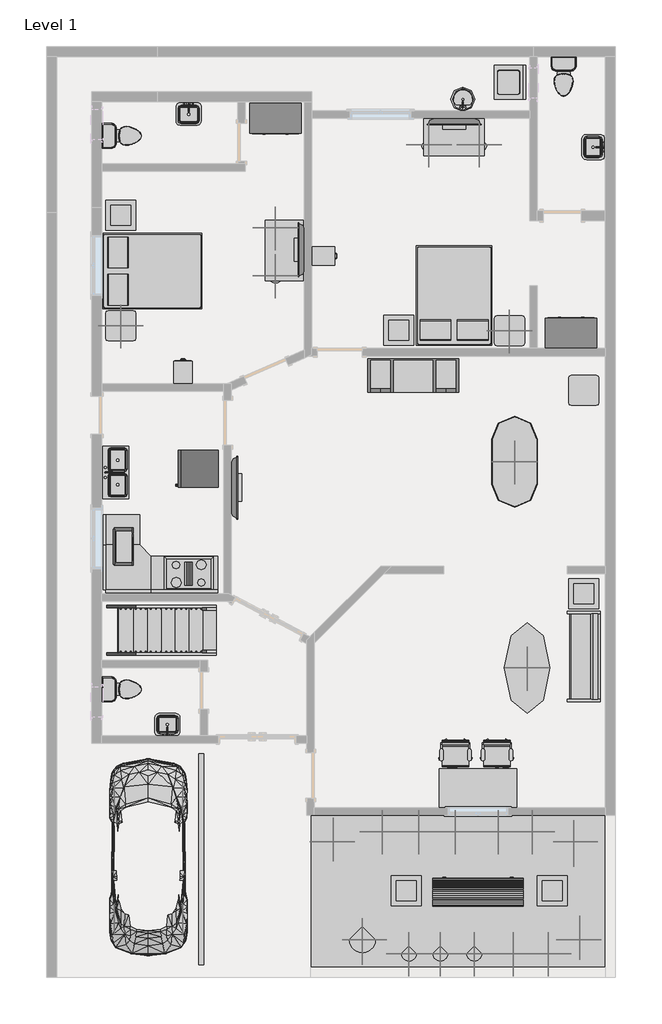
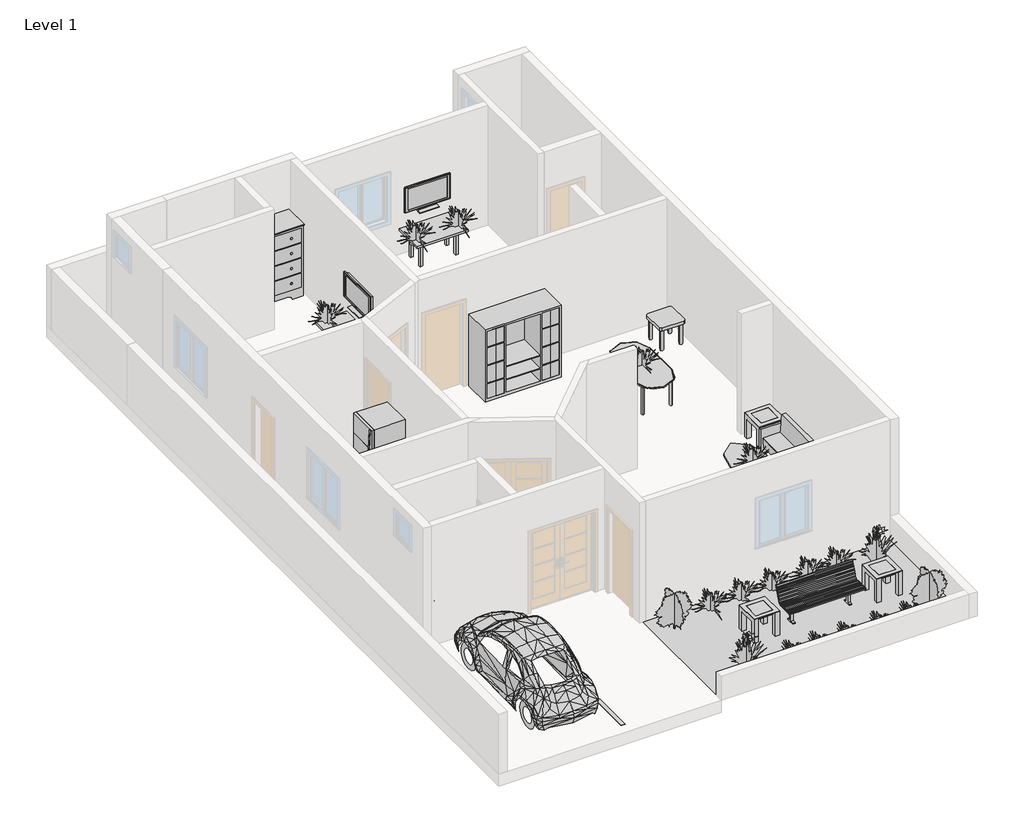
# One storey, part 2 of 2: 27 furniture elements, 23 geographic elements, 12 flow terminals, 7 proxies, 2 members, 2 railings, 1 stair flight.
"""IFC4 building model written with IfcOpenShell, lengths in millimetres."""

from ifc_helpers import new_model, si_unit, frame, origin, place, context, project, spatial, polyline, outline, extrude, triangles, transform, mapped, element, save
from components import proxy_bb1e6e30, proxy_8a8d5ab2, parking_space_9_x_18_90_deg_fdd9e8f5, rpc_beetle_rpc_beetle_3ce7ba48, proxy_a13a33b2, proxy_718fa39f, flow_terminal_accce45a, flow_terminal_a53be723, flow_terminal_d49f872f, flow_terminal_62a433f7, toilet_domestic_3d_toilet_domestic_3d_f7549cf7, toilet_domestic_3d_toilet_domestic_3d_183bbd19, furniture_1d2926bd, furniture_bb55ed6b, chair_task_arms_chair_task_arms_fa5a08ef, furniture_072f6425, furniture_f72bdee3, furniture_cf0b6580, furniture_a4ffab56, furniture_7a3aaa4f, furniture_fdf74506, furniture_b5c51a22, furniture_2c34a4f9, furniture_962d0db1, furniture_31d08a24, furniture_3f969c1c, furniture_b52c1e80, geographic_element_235d1464, rpc_plant_tropical_55f6ff97, rpc_plant_tropical_agave_1_5_93a2a214, rpc_plant_tropical_jungle_flame_3_9c4808c2, stair_flight_e425de01

model = new_model("IFC4")

# Units and contexts
model_context = context("Model", 3, world=origin())
ifc_project = project(units=[si_unit("LENGTHUNIT", "METRE", prefix="MILLI")], contexts=[model_context])

# Site, building, storey
site = spatial("IfcSite", under=ifc_project)
building = spatial("IfcBuilding", under=site)
storey = spatial("IfcBuildingStorey", under=building, Name="Level 1", Elevation=0.0)

# Proxies
placement = place(None, origin())
element("IfcBuildingElementProxy", 1, Name="Building Element Proxy", at=placement, inside=storey, context=model_context, shape_type="Tessellation", body=[
    triangles([(-7577.7508347, -2699.6256248, 0.0), (-7501.5508347, -5773.025528, 0.0), (-1557.950544, -5773.025528, 0.0), (-1557.950544, -2699.6256248, 0.0)], [[1, 2, 4], [3, 4, 2]], closed=False),
])
proxy_shape = proxy_bb1e6e30(model_context)
element("IfcBuildingElementProxy", 2, Name="Cook Top-4 Unit : 36\" x 20\"", ObjectType="Cook Top-4 Unit : 36\" x 20\"", at=placement, inside=storey, context=model_context, shape_type="MappedRepresentation", body=[
    mapped(proxy_shape, transform((-9965.3505662, 2175.4598603, 0.0), x_axis=(1.0, 0.0, 0.0), y_axis=(0.0, 1.0, 0.0), z_axis=(0.0, 0.0, 1.0))),
])
proxy_2_shape = proxy_8a8d5ab2(model_context)
element("IfcBuildingElementProxy", 3, Name="Microwave : 30\" x 16\" x 18\"", ObjectType="Microwave : 30\" x 16\" x 18\"", at=placement, inside=storey, context=model_context, shape_type="MappedRepresentation", body=[
    mapped(proxy_2_shape, transform((-11639.231072, 2222.1807348, 0.0), x_axis=(0.0, 1.0000000000000004, 0.0), y_axis=(-1.0000000000000004, 0.0, 0.0), z_axis=(0.0, 0.0, 1.0))),
])
parking_space_9_x_18_90_deg_shape = parking_space_9_x_18_90_deg_fdd9e8f5(model_context)
element("IfcBuildingElementProxy", 4, Name="Parking Space : 9' x 18' - 90 deg", ObjectType="Parking Space : 9' x 18' - 90 deg", at=placement, inside=storey, context=model_context, shape_type="MappedRepresentation", body=[
    mapped(parking_space_9_x_18_90_deg_shape, transform((-9711.3505662, -5722.2257293, 0.0), x_axis=(-1.0, 0.0, 0.0), y_axis=(0.0, -1.0, 0.0), z_axis=(0.0, 0.0, 1.0))),
])
rpc_beetle_rpc_beetle_shape = rpc_beetle_rpc_beetle_3ce7ba48(model_context)
element("IfcBuildingElementProxy", 5, Name="RPC Beetle : RPC Beetle", ObjectType="RPC Beetle : RPC Beetle", at=placement, inside=storey, context=model_context, shape_type="MappedRepresentation", body=[
    mapped(rpc_beetle_rpc_beetle_shape, transform((-10778.1505662, -4782.4257293, 0.0), x_axis=(1.0, 0.0, 0.0), y_axis=(0.0, 1.0, 0.0), z_axis=(0.0, 0.0, 1.0))),
])
proxy_3_shape = proxy_a13a33b2(model_context)
element("IfcBuildingElementProxy", 6, Name="Refrigerator : 30\" x 32\" RH", ObjectType="Refrigerator : 30\" x 32\" RH", at=placement, inside=storey, context=model_context, shape_type="MappedRepresentation", body=[
    mapped(proxy_3_shape, transform((-9754.2130662, 4296.8752993, 0.0), x_axis=(0.0, -1.0000000000000007, 0.0), y_axis=(1.0000000000000007, 0.0, 0.0), z_axis=(0.0, 0.0, 1.0))),
])
proxy_4_shape = proxy_718fa39f(model_context)
element("IfcBuildingElementProxy", 7, Name="Washer : 27\" x 25\" x 35\"", ObjectType="Washer : 27\" x 25\" x 35\"", at=placement, inside=storey, context=model_context, shape_type="MappedRepresentation", body=[
    mapped(proxy_4_shape, transform((-3754.800131, 12516.2917392, 0.0), x_axis=(0.0, -1.0000000000000004, 0.0), y_axis=(1.0000000000000004, 0.0, 0.0), z_axis=(0.0, 0.0, 1.0))),
])

# Flow terminals
flow_terminal_shape = flow_terminal_accce45a(model_context)
element("IfcFlowTerminal", 8, ObjectType="Floor Drain - Round : 5\" Strainer - 2\" Drain", at=placement, inside=storey, context=model_context, shape_type="MappedRepresentation", body=[
    mapped(flow_terminal_shape, transform((-10955.9505662, 11498.9742707, 0.0), x_axis=(1.0, 0.0, 0.0), y_axis=(0.0, 1.0, 0.0), z_axis=(0.0, 0.0, 1.0))),
])
element("IfcFlowTerminal", 9, ObjectType="Floor Drain - Round : 5\" Strainer - 2\" Drain", at=placement, inside=storey, context=model_context, shape_type="MappedRepresentation", body=[
    mapped(flow_terminal_shape, transform((-1938.9505662, 11727.5742707, 0.0), x_axis=(1.0, 0.0, 0.0), y_axis=(0.0, 1.0, 0.0), z_axis=(0.0, 0.0, 1.0))),
])
element("IfcFlowTerminal", 10, ObjectType="Floor Drain - Round : 5\" Strainer - 2\" Drain", at=placement, inside=storey, context=model_context, shape_type="MappedRepresentation", body=[
    mapped(flow_terminal_shape, transform((-11438.5505662, -743.8257293, 0.0), x_axis=(1.0, 0.0, 0.0), y_axis=(0.0, 1.0, 0.0), z_axis=(0.0, 0.0, 1.0))),
])
element("IfcFlowTerminal", 11, ObjectType="Floor Drain - Round : 5\" Strainer - 2\" Drain", at=placement, inside=storey, context=model_context, shape_type="MappedRepresentation", body=[
    mapped(flow_terminal_shape, transform((-4072.5505662, 12413.3742707, 0.0), x_axis=(1.0, 0.0, 0.0), y_axis=(0.0, 1.0, 0.0), z_axis=(0.0, 0.0, 1.0))),
])
flow_terminal_2_shape = flow_terminal_a53be723(model_context)
element("IfcFlowTerminal", 12, ObjectType="Sink Kitchen-Double : 42\" x 21\"", at=placement, inside=storey, context=model_context, shape_type="MappedRepresentation", body=[
    mapped(flow_terminal_2_shape, transform((-11436.2051651, 4204.4706197, 0.0), x_axis=(0.0, 1.0000000000000002, 0.0), y_axis=(-1.0000000000000002, 0.0, 0.0), z_axis=(0.0, 0.0, 1.0))),
])
flow_terminal_3_shape = flow_terminal_d49f872f(model_context)
element("IfcFlowTerminal", 13, ObjectType="Sink Vanity-Round : 19\" x 19\"", at=placement, inside=storey, context=model_context, shape_type="MappedRepresentation", body=[
    mapped(flow_terminal_3_shape, transform((-4331.4988256, 11839.263255, 0.0), x_axis=(-1.0000000000000004, 0.0, 0.0), y_axis=(0.0, -1.0000000000000004, 0.0), z_axis=(0.0, 0.0, 1.0))),
])
flow_terminal_4_shape = flow_terminal_62a433f7(model_context)
element("IfcFlowTerminal", 14, ObjectType="Sink Vanity-Square : 20\" x 18\"", at=placement, inside=storey, context=model_context, shape_type="MappedRepresentation", body=[
    mapped(flow_terminal_4_shape, transform((-9981.0398067, 11502.9788696, 0.0), x_axis=(1.0, 0.0, 0.0), y_axis=(0.0, 1.0, 0.0), z_axis=(0.0, 0.0, 1.0))),
])
element("IfcFlowTerminal", 15, ObjectType="Sink Vanity-Square : 20\" x 18\"", at=placement, inside=storey, context=model_context, shape_type="MappedRepresentation", body=[
    mapped(flow_terminal_4_shape, transform((-1750.7959673, 10803.4635113, 0.0), x_axis=(0.0, -1.0000000000000002, 0.0), y_axis=(1.0000000000000002, 0.0, 0.0), z_axis=(0.0, 0.0, 1.0))),
])
element("IfcFlowTerminal", 16, ObjectType="Sink Vanity-Square : 20\" x 18\"", at=placement, inside=storey, context=model_context, shape_type="MappedRepresentation", body=[
    mapped(flow_terminal_4_shape, transform((-10381.4613256, -919.2803281, 0.0), x_axis=(-1.0, 0.0, 0.0), y_axis=(0.0, -1.0, 0.0), z_axis=(0.0, 0.0, 1.0))),
])
toilet_domestic_3d_toilet_domestic_3d_shape = toilet_domestic_3d_toilet_domestic_3d_f7549cf7(model_context)
toilet_domestic_3d_toilet_domestic_3d_2_shape = toilet_domestic_3d_toilet_domestic_3d_183bbd19(model_context)
element("IfcFlowTerminal", 17, ObjectType="Toilet-Domestic-3D : Toilet-Domestic-3D", at=placement, inside=storey, context=model_context, shape_type="MappedRepresentation", body=[
    mapped(toilet_domestic_3d_toilet_domestic_3d_shape, transform((-11223.2545388, 11016.3742707, 0.0), x_axis=(0.0, 1.0, 0.0), y_axis=(-1.0, 0.0, 0.0), z_axis=(0.0, 0.0, 1.0))),
    mapped(toilet_domestic_3d_toilet_domestic_3d_2_shape, transform((-11223.2545388, 11016.3742707, 0.0), x_axis=(0.0, 1.0, 0.0), y_axis=(-1.0, 0.0, 0.0), z_axis=(0.0, 0.0, 1.0))),
])
element("IfcFlowTerminal", 18, ObjectType="Toilet-Domestic-3D : Toilet-Domestic-3D", at=placement, inside=storey, context=model_context, shape_type="MappedRepresentation", body=[
    mapped(toilet_domestic_3d_toilet_domestic_3d_shape, transform((-2396.1505662, 12121.8782434, 0.0), x_axis=(1.0, 0.0, 0.0), y_axis=(0.0, 1.0, 0.0), z_axis=(0.0, 0.0, 1.0))),
    mapped(toilet_domestic_3d_toilet_domestic_3d_2_shape, transform((-2396.1505662, 12121.8782434, 0.0), x_axis=(1.0, 0.0, 0.0), y_axis=(0.0, 1.0, 0.0), z_axis=(0.0, 0.0, 1.0))),
])
element("IfcFlowTerminal", 19, ObjectType="Toilet-Domestic-3D : Toilet-Domestic-3D", at=placement, inside=storey, context=model_context, shape_type="MappedRepresentation", body=[
    mapped(toilet_domestic_3d_toilet_domestic_3d_shape, transform((-11223.2545388, -159.6257293, 0.0), x_axis=(0.0, 1.0000000000000002, 0.0), y_axis=(-1.0000000000000002, 0.0, 0.0), z_axis=(0.0, 0.0, 1.0))),
    mapped(toilet_domestic_3d_toilet_domestic_3d_2_shape, transform((-11223.2545388, -159.6257293, 0.0), x_axis=(0.0, 1.0000000000000002, 0.0), y_axis=(-1.0000000000000002, 0.0, 0.0), z_axis=(0.0, 0.0, 1.0))),
])

# Furniture
furniture_shape = furniture_1d2926bd(model_context)
element("IfcFurniture", 20, ObjectType="Bed-Box : Queen 60\" x 79\"", at=placement, inside=storey, context=model_context, shape_type="MappedRepresentation", body=[
    mapped(furniture_shape, transform((-10936.3800744, 7946.7218117, 0.0), x_axis=(0.0, 1.0, 0.0), y_axis=(-1.0, 0.0, 0.0), z_axis=(0.0, 0.0, 1.0))),
])
element("IfcFurniture", 21, ObjectType="Bed-Box : Queen 60\" x 79\"", at=placement, inside=storey, context=model_context, shape_type="MappedRepresentation", body=[
    mapped(furniture_shape, transform((-4266.7981072, 7556.1772543, 0.0), x_axis=(-1.0, 0.0, 0.0), y_axis=(0.0, -1.0, 0.0), z_axis=(0.0, 0.0, 1.0))),
])
furniture_2_shape = furniture_bb55ed6b(model_context)
element("IfcFurniture", 22, ObjectType="Cabinet-File 2 Drawer : 15\" x 18\"", at=placement, inside=storey, context=model_context, shape_type="MappedRepresentation", body=[
    mapped(furniture_2_shape, transform((-10207.5470132, 6097.3255602, 0.0), x_axis=(-1.0, 0.0, 0.0), y_axis=(0.0, -1.0, 0.0), z_axis=(0.0, 0.0, 1.0))),
])
element("IfcFurniture", 23, ObjectType="Cabinet-File 2 Drawer : 15\" x 18\"", at=placement, inside=storey, context=model_context, shape_type="MappedRepresentation", body=[
    mapped(furniture_2_shape, transform((-7389.6848663, 8718.5707178, 0.0), x_axis=(0.0, 1.0000000000000002, 0.0), y_axis=(-1.0000000000000002, 0.0, 0.0), z_axis=(0.0, 0.0, 1.0))),
])
chair_task_arms_chair_task_arms_shape = chair_task_arms_chair_task_arms_fa5a08ef(model_context)
element("IfcFurniture", 24, ObjectType="Chair-Task Arms : Chair-Task Arms", at=placement, inside=storey, context=model_context, shape_type="MappedRepresentation", body=[
    mapped(chair_task_arms_chair_task_arms_shape, transform((-4439.5597465, -1436.0798276, 0.0), x_axis=(-1.0000000000000004, 0.0, 0.0), y_axis=(0.0, -1.0000000000000004, 0.0), z_axis=(0.0, 0.0, 1.0))),
])
element("IfcFurniture", 25, ObjectType="Chair-Task Arms : Chair-Task Arms", at=placement, inside=storey, context=model_context, shape_type="MappedRepresentation", body=[
    mapped(chair_task_arms_chair_task_arms_shape, transform((-3601.3597465, -1436.0798276, 0.0), x_axis=(-1.0000000000000004, 0.0, 0.0), y_axis=(0.0, -1.0000000000000004, 0.0), z_axis=(0.0, 0.0, 1.0))),
])
furniture_3_shape = furniture_072f6425(model_context)
element("IfcFurniture", 26, ObjectType="Desk : 60\" x 30\" Student", at=placement, inside=storey, context=model_context, shape_type="MappedRepresentation", body=[
    mapped(furniture_3_shape, transform((-4885.3505662, -2547.2257293, 0.0), x_axis=(1.0, 0.0, 0.0), y_axis=(0.0, 1.0, 0.0), z_axis=(0.0, 0.0, 1.0))),
])
furniture_4_shape = furniture_f72bdee3(model_context)
element("IfcFurniture", 27, ObjectType="Dresser : 48\" x 72\" x 24\"", at=placement, inside=storey, context=model_context, shape_type="MappedRepresentation", body=[
    mapped(furniture_4_shape, transform((-7943.5573063, 11735.1372248, 0.0), x_axis=(1.0, 0.0, 0.0), y_axis=(0.0, 1.0, 0.0), z_axis=(0.0, 0.0, 1.0))),
])
element("IfcFurniture", 28, ObjectType="Dresser : 48\" x 72\" x 24\"", at=placement, inside=storey, context=model_context, shape_type="MappedRepresentation", body=[
    mapped(furniture_4_shape, transform((-2512.943826, 6665.4113166, 0.0), x_axis=(-1.0000000000000004, 0.0, 0.0), y_axis=(0.0, -1.0000000000000004, 0.0), z_axis=(0.0, 0.0, 1.0))),
])
furniture_5_shape = furniture_cf0b6580(model_context)
element("IfcFurniture", 29, ObjectType="Entertainment Center : 72\" x 72\" x 24\"", at=placement, inside=storey, context=model_context, shape_type="MappedRepresentation", body=[
    mapped(furniture_5_shape, transform((-5431.4505662, 6620.4598603, 0.0), x_axis=(1.0, 0.0, 0.0), y_axis=(0.0, 1.0, 0.0), z_axis=(0.0, 0.0, 1.0))),
])
furniture_6_shape = furniture_a4ffab56(model_context)
element("IfcFurniture", 30, ObjectType="Sofa : 72\"", at=placement, inside=storey, context=model_context, shape_type="MappedRepresentation", body=[
    mapped(furniture_6_shape, transform((-2135.9046645, 571.1447625, 0.0), x_axis=(0.0, -1.0, 0.0), y_axis=(1.0, 0.0, 0.0), z_axis=(0.0, 0.0, 1.0))),
])
furniture_7_shape = furniture_7a3aaa4f(model_context)
element("IfcFurniture", 31, ObjectType="TV - Flat Screen : 42\"", at=placement, inside=storey, context=model_context, shape_type="MappedRepresentation", body=[
    mapped(furniture_7_shape, transform((-7687.0891898, 8713.7297566, 1041.4), x_axis=(0.0, -1.0000000000000002, 0.0), y_axis=(1.0000000000000002, 0.0, 0.0), z_axis=(0.0, 0.0, 1.0))),
])
element("IfcFurniture", 32, ObjectType="TV - Flat Screen : 42\"", at=placement, inside=storey, context=model_context, shape_type="MappedRepresentation", body=[
    mapped(furniture_7_shape, transform((-4602.006052, 11305.3729828, 1041.4), x_axis=(1.0, 0.0, 0.0), y_axis=(0.0, 1.0, 0.0), z_axis=(0.0, 0.0, 1.0))),
])
furniture_8_shape = furniture_fdf74506(model_context)
element("IfcFurniture", 33, ObjectType="TV - Flat Screen : 50\"", at=placement, inside=storey, context=model_context, shape_type="MappedRepresentation", body=[
    mapped(furniture_8_shape, transform((-9043.2119425, 3917.352407, 1041.4), x_axis=(0.0, 1.0, 0.0), y_axis=(-1.0, 0.0, 0.0), z_axis=(0.0, 0.0, 1.0))),
])
furniture_9_shape = furniture_b5c51a22(model_context)
element("IfcFurniture", 34, ObjectType="Table-Coffee : 24\" x 24\" x 24\"", at=placement, inside=storey, context=model_context, shape_type="MappedRepresentation", body=[
    mapped(furniture_9_shape, transform((-11355.2163328, 9320.9631929, 0.0), x_axis=(1.0, 0.0, 0.0), y_axis=(0.0, 1.0, 0.0), z_axis=(0.0, 0.0, 1.0))),
])
element("IfcFurniture", 35, ObjectType="Table-Coffee : 24\" x 24\" x 24\"", at=placement, inside=storey, context=model_context, shape_type="MappedRepresentation", body=[
    mapped(furniture_9_shape, transform((-5741.8163328, 6996.8956847, 0.0), x_axis=(1.0, 0.0, 0.0), y_axis=(0.0, 1.0, 0.0), z_axis=(0.0, 0.0, 1.0))),
])
element("IfcFurniture", 36, ObjectType="Table-Coffee : 24\" x 24\" x 24\"", at=placement, inside=storey, context=model_context, shape_type="MappedRepresentation", body=[
    mapped(furniture_9_shape, transform((-2008.0163328, 1673.8487825, 0.0), x_axis=(1.0, 0.0, 0.0), y_axis=(0.0, 1.0, 0.0), z_axis=(0.0, 0.0, 1.0))),
])
element("IfcFurniture", 37, ObjectType="Table-Coffee : 24\" x 24\" x 24\"", at=placement, inside=storey, context=model_context, shape_type="MappedRepresentation", body=[
    mapped(furniture_9_shape, transform((-2643.0163328, -4318.8368071, 0.0), x_axis=(1.0, 0.0, 0.0), y_axis=(0.0, 1.0, 0.0), z_axis=(0.0, 0.0, 1.0))),
])
element("IfcFurniture", 38, ObjectType="Table-Coffee : 24\" x 24\" x 24\"", at=placement, inside=storey, context=model_context, shape_type="MappedRepresentation", body=[
    mapped(furniture_9_shape, transform((-5589.4163328, -4318.8368071, 0.0), x_axis=(1.0, 0.0, 0.0), y_axis=(0.0, 1.0, 0.0), z_axis=(0.0, 0.0, 1.0))),
])
furniture_10_shape = furniture_2c34a4f9(model_context)
element("IfcFurniture", 39, ObjectType="Table-Dining Oval : 36\" x 72\"", at=placement, inside=storey, context=model_context, shape_type="MappedRepresentation", body=[
    mapped(furniture_10_shape, transform((-3028.6522055, 4034.2401882, 0.0), x_axis=(0.0, -0.9999999999999998, 0.0), y_axis=(0.9999999999999998, 0.0, 0.0), z_axis=(0.0, 0.0, 1.0))),
])
furniture_11_shape = furniture_962d0db1(model_context)
element("IfcFurniture", 40, ObjectType="Table-Ellipse : 72\" x 36\"", at=placement, inside=storey, context=model_context, shape_type="MappedRepresentation", body=[
    mapped(furniture_11_shape, transform((-3132.7505662, 272.1742707, 0.0), x_axis=(0.0, 1.0, 0.0), y_axis=(-1.0, 0.0, 0.0), z_axis=(0.0, 0.0, 1.0))),
])
furniture_12_shape = furniture_31d08a24(model_context)
element("IfcFurniture", 41, ObjectType="Table-End : 24\" x 24\"", at=placement, inside=storey, context=model_context, shape_type="MappedRepresentation", body=[
    mapped(furniture_12_shape, transform((-11645.4841965, 7028.5742707, 0.0), x_axis=(1.0, 0.0, 0.0), y_axis=(0.0, 1.0, 0.0), z_axis=(0.0, 0.0, 1.0))),
])
element("IfcFurniture", 42, ObjectType="Table-End : 24\" x 24\"", at=placement, inside=storey, context=model_context, shape_type="MappedRepresentation", body=[
    mapped(furniture_12_shape, transform((-3796.8841965, 6927.0067625, 0.0), x_axis=(1.0, 0.0, 0.0), y_axis=(0.0, 1.0, 0.0), z_axis=(0.0, 0.0, 1.0))),
])
element("IfcFurniture", 43, ObjectType="Table-End : 24\" x 24\"", at=placement, inside=storey, context=model_context, shape_type="MappedRepresentation", body=[
    mapped(furniture_12_shape, transform((-2298.2841965, 5725.1098603, 0.0), x_axis=(1.0, 0.0, 0.0), y_axis=(0.0, 1.0, 0.0), z_axis=(0.0, 0.0, 1.0))),
])
furniture_13_shape = furniture_3f969c1c(model_context)
element("IfcFurniture", 44, ObjectType="Table-Rectangular : 72\" x 30\"", at=placement, inside=storey, context=model_context, shape_type="MappedRepresentation", body=[
    mapped(furniture_13_shape, transform((-8034.9505662, 8704.9742707, 0.0), x_axis=(0.0, 1.0000000000000002, 0.0), y_axis=(-1.0000000000000002, 0.0, 0.0), z_axis=(0.0, 0.0, 1.0))),
])
element("IfcFurniture", 45, ObjectType="Table-Rectangular : 72\" x 30\"", at=placement, inside=storey, context=model_context, shape_type="MappedRepresentation", body=[
    mapped(furniture_13_shape, transform((-4605.9505662, 10990.9742707, 0.0), x_axis=(1.0, 0.0, 0.0), y_axis=(0.0, 1.0, 0.0), z_axis=(0.0, 0.0, 1.0))),
])
furniture_14_shape = furniture_b52c1e80(model_context)
element("IfcFurniture", 46, ObjectType="Work Station Cubicle : 96\" x 96\"", at=placement, inside=storey, context=model_context, shape_type="MappedRepresentation", body=[
    mapped(furniture_14_shape, transform((-12187.5735738, 1927.906023, 0.0), x_axis=(0.0, 0.9999999999999999, 0.0), y_axis=(-0.9999999999999999, 0.0, 0.0), z_axis=(0.0, 0.0, 1.0))),
])

# Geographic elements
geographic_element_shape = geographic_element_235d1464(model_context)
element("IfcGeographicElement", 47, ObjectType="Park Bench : 72\"", at=placement, inside=storey, context=model_context, shape_type="MappedRepresentation", body=[
    mapped(geographic_element_shape, transform((-4123.3505662, -4223.6257293, 0.0), x_axis=(1.0, 0.0, 0.0), y_axis=(0.0, 1.0, 0.0), z_axis=(0.0, 0.0, 1.0))),
])
rpc_plant_tropical_shape = rpc_plant_tropical_55f6ff97(model_context)
element("IfcGeographicElement", 48, ObjectType="RPC Plant - Tropical", at=placement, inside=storey, context=model_context, shape_type="MappedRepresentation", body=[
    mapped(rpc_plant_tropical_shape, transform((-6460.1505662, -5214.2257293, 0.0), x_axis=(1.0, 0.0, 0.0), y_axis=(0.0, 1.0, 0.0), z_axis=(0.0, 0.0, 1.0))),
])
element("IfcGeographicElement", 49, ObjectType="RPC Plant - Tropical", at=placement, inside=storey, context=model_context, shape_type="MappedRepresentation", body=[
    mapped(rpc_plant_tropical_shape, transform((-2192.9505662, -3233.0257293, 0.0), x_axis=(1.0, 0.0, 0.0), y_axis=(0.0, 1.0, 0.0), z_axis=(0.0, 0.0, 1.0))),
])
rpc_plant_tropical_agave_1_5_shape = rpc_plant_tropical_agave_1_5_93a2a214(model_context)
element("IfcGeographicElement", 50, ObjectType="RPC Plant - Tropical : Agave - 1.5'", at=placement, inside=storey, context=model_context, shape_type="MappedRepresentation", body=[
    mapped(rpc_plant_tropical_agave_1_5_shape, transform((-11336.9505662, 7180.9742707, 609.6), x_axis=(1.0, 0.0, 0.0), y_axis=(0.0, 1.0, 0.0), z_axis=(0.0, 0.0, 1.0))),
])
element("IfcGeographicElement", 51, ObjectType="RPC Plant - Tropical : Agave - 1.5'", at=placement, inside=storey, context=model_context, shape_type="MappedRepresentation", body=[
    mapped(rpc_plant_tropical_agave_1_5_shape, transform((-8212.7505662, 8196.9742707, 660.4), x_axis=(1.0, 0.0, 0.0), y_axis=(0.0, 1.0, 0.0), z_axis=(0.0, 0.0, 1.0))),
])
element("IfcGeographicElement", 52, ObjectType="RPC Plant - Tropical : Agave - 1.5'", at=placement, inside=storey, context=model_context, shape_type="MappedRepresentation", body=[
    mapped(rpc_plant_tropical_agave_1_5_shape, transform((-8212.7505662, 9162.1742707, 660.4), x_axis=(1.0, 0.0, 0.0), y_axis=(0.0, 1.0, 0.0), z_axis=(0.0, 0.0, 1.0))),
])
element("IfcGeographicElement", 53, ObjectType="RPC Plant - Tropical : Agave - 1.5'", at=placement, inside=storey, context=model_context, shape_type="MappedRepresentation", body=[
    mapped(rpc_plant_tropical_agave_1_5_shape, transform((-3488.3505662, 7079.4067625, 609.6), x_axis=(1.0, 0.0, 0.0), y_axis=(0.0, 1.0, 0.0), z_axis=(0.0, 0.0, 1.0))),
])
element("IfcGeographicElement", 54, ObjectType="RPC Plant - Tropical : Agave - 1.5'", at=placement, inside=storey, context=model_context, shape_type="MappedRepresentation", body=[
    mapped(rpc_plant_tropical_agave_1_5_shape, transform((-5113.9505662, 10838.5742707, 609.6), x_axis=(1.0, 0.0, 0.0), y_axis=(0.0, 1.0, 0.0), z_axis=(0.0, 0.0, 1.0))),
])
element("IfcGeographicElement", 55, ObjectType="RPC Plant - Tropical : Agave - 1.5'", at=placement, inside=storey, context=model_context, shape_type="MappedRepresentation", body=[
    mapped(rpc_plant_tropical_agave_1_5_shape, transform((-4097.9505662, 10838.5742707, 609.6), x_axis=(1.0, 0.0, 0.0), y_axis=(0.0, 1.0, 0.0), z_axis=(0.0, 0.0, 1.0))),
])
element("IfcGeographicElement", 56, ObjectType="RPC Plant - Tropical : Agave - 1.5'", at=placement, inside=storey, context=model_context, shape_type="MappedRepresentation", body=[
    mapped(rpc_plant_tropical_agave_1_5_shape, transform((-3132.7505662, 272.1742707, 660.4), x_axis=(1.0, 0.0, 0.0), y_axis=(0.0, 1.0, 0.0), z_axis=(0.0, 0.0, 1.0))),
])
element("IfcGeographicElement", 57, ObjectType="RPC Plant - Tropical : Agave - 1.5'", at=placement, inside=storey, context=model_context, shape_type="MappedRepresentation", body=[
    mapped(rpc_plant_tropical_agave_1_5_shape, transform((-3386.7505662, 4436.0598603, 685.8), x_axis=(1.0, 0.0, 0.0), y_axis=(0.0, 1.0, 0.0), z_axis=(0.0, 0.0, 1.0))),
])
element("IfcGeographicElement", 58, ObjectType="RPC Plant - Tropical : Agave - 1.5'", at=placement, inside=storey, context=model_context, shape_type="MappedRepresentation", body=[
    mapped(rpc_plant_tropical_agave_1_5_shape, transform((-6053.7505662, -3029.8257293, 0.0), x_axis=(1.0, 0.0, 0.0), y_axis=(0.0, 1.0, 0.0), z_axis=(0.0, 0.0, 1.0))),
])
element("IfcGeographicElement", 59, ObjectType="RPC Plant - Tropical : Agave - 1.5'", at=placement, inside=storey, context=model_context, shape_type="MappedRepresentation", body=[
    mapped(rpc_plant_tropical_agave_1_5_shape, transform((-3031.1505662, -3029.8257293, 0.0), x_axis=(1.0, 0.0, 0.0), y_axis=(0.0, 1.0, 0.0), z_axis=(0.0, 0.0, 1.0))),
])
element("IfcGeographicElement", 60, ObjectType="RPC Plant - Tropical : Agave - 1.5'", at=placement, inside=storey, context=model_context, shape_type="MappedRepresentation", body=[
    mapped(rpc_plant_tropical_agave_1_5_shape, transform((-2700.9505662, -5493.6257293, 0.0), x_axis=(1.0, 0.0, 0.0), y_axis=(0.0, 1.0, 0.0), z_axis=(0.0, 0.0, 1.0))),
])
element("IfcGeographicElement", 61, ObjectType="RPC Plant - Tropical : Agave - 1.5'", at=placement, inside=storey, context=model_context, shape_type="MappedRepresentation", body=[
    mapped(rpc_plant_tropical_agave_1_5_shape, transform((-3412.1505662, -5493.6257293, 0.0), x_axis=(1.0, 0.0, 0.0), y_axis=(0.0, 1.0, 0.0), z_axis=(0.0, 0.0, 1.0))),
])
element("IfcGeographicElement", 62, ObjectType="RPC Plant - Tropical : Agave - 1.5'", at=placement, inside=storey, context=model_context, shape_type="MappedRepresentation", body=[
    mapped(rpc_plant_tropical_agave_1_5_shape, transform((-4199.5505662, -5493.6257293, 0.0), x_axis=(1.0, 0.0, 0.0), y_axis=(0.0, 1.0, 0.0), z_axis=(0.0, 0.0, 1.0))),
])
element("IfcGeographicElement", 63, ObjectType="RPC Plant - Tropical : Agave - 1.5'", at=placement, inside=storey, context=model_context, shape_type="MappedRepresentation", body=[
    mapped(rpc_plant_tropical_agave_1_5_shape, transform((-4885.3505662, -5493.6257293, 0.0), x_axis=(1.0, 0.0, 0.0), y_axis=(0.0, 1.0, 0.0), z_axis=(0.0, 0.0, 1.0))),
])
element("IfcGeographicElement", 64, ObjectType="RPC Plant - Tropical : Agave - 1.5'", at=placement, inside=storey, context=model_context, shape_type="MappedRepresentation", body=[
    mapped(rpc_plant_tropical_agave_1_5_shape, transform((-5520.3505662, -5493.6257293, 0.0), x_axis=(1.0, 0.0, 0.0), y_axis=(0.0, 1.0, 0.0), z_axis=(0.0, 0.0, 1.0))),
])
element("IfcGeographicElement", 65, ObjectType="RPC Plant - Tropical : Agave - 1.5'", at=placement, inside=storey, context=model_context, shape_type="MappedRepresentation", body=[
    mapped(rpc_plant_tropical_agave_1_5_shape, transform((-5317.1505662, -3029.8257293, 0.0), x_axis=(1.0, 0.0, 0.0), y_axis=(0.0, 1.0, 0.0), z_axis=(0.0, 0.0, 1.0))),
])
element("IfcGeographicElement", 66, ObjectType="RPC Plant - Tropical : Agave - 1.5'", at=placement, inside=storey, context=model_context, shape_type="MappedRepresentation", body=[
    mapped(rpc_plant_tropical_agave_1_5_shape, transform((-4580.5505662, -3029.8257293, 0.0), x_axis=(1.0, 0.0, 0.0), y_axis=(0.0, 1.0, 0.0), z_axis=(0.0, 0.0, 1.0))),
])
element("IfcGeographicElement", 67, ObjectType="RPC Plant - Tropical : Agave - 1.5'", at=placement, inside=storey, context=model_context, shape_type="MappedRepresentation", body=[
    mapped(rpc_plant_tropical_agave_1_5_shape, transform((-3716.9505662, -3029.8257293, 0.0), x_axis=(1.0, 0.0, 0.0), y_axis=(0.0, 1.0, 0.0), z_axis=(0.0, 0.0, 1.0))),
])
rpc_plant_tropical_jungle_flame_3_shape = rpc_plant_tropical_jungle_flame_3_9c4808c2(model_context)
element("IfcGeographicElement", 68, ObjectType="RPC Plant - Tropical : Jungle Flame - 3'", at=placement, inside=storey, context=model_context, shape_type="MappedRepresentation", body=[
    mapped(rpc_plant_tropical_jungle_flame_3_shape, transform((-7044.3505662, -3233.0257293, 0.0), x_axis=(1.0, 0.0, 0.0), y_axis=(0.0, 1.0, 0.0), z_axis=(0.0, 0.0, 1.0))),
])
element("IfcGeographicElement", 69, ObjectType="RPC Plant - Tropical : Jungle Flame - 3'", at=placement, inside=storey, context=model_context, shape_type="MappedRepresentation", body=[
    mapped(rpc_plant_tropical_jungle_flame_3_shape, transform((-2065.9505662, -5214.2257293, 0.0), x_axis=(1.0, 0.0, 0.0), y_axis=(0.0, 1.0, 0.0), z_axis=(0.0, 0.0, 1.0))),
])

# Members
element("IfcMember", 70, ObjectType="Stringer - 2\" Width", at=placement, inside=storey, context=model_context, shape_type="SweptSolid", body=[
    extrude(outline(polyline([(0.0, -9406.5505662), (212.114512, -9406.5505662), (1566.7811786, -11641.7505662), (1210.3724171, -11641.7505662), (0.0, -9644.6360779), (0.0, -9406.5505662)])), frame((0.0, 526.1742707, 0.0), z_axis=(0.0, 1.0, 0.0), x_axis=(0.0, 0.0, 1.0)), (0.0, 0.0, 1.0), 50.8),
])
element("IfcMember", 71, ObjectType="Stringer - 2\" Width", at=placement, inside=storey, context=model_context, shape_type="SweptSolid", body=[
    extrude(outline(polyline([(0.0, -9406.5505662), (212.114512, -9406.5505662), (1566.7811786, -11641.7505662), (1210.3724171, -11641.7505662), (0.0, -9644.6360779), (0.0, -9406.5505662)])), frame((0.0, 1491.3742707, 0.0), z_axis=(0.0, 1.0, 0.0), x_axis=(0.0, 0.0, 1.0)), (0.0, 0.0, 1.0), 50.8),
])

# Railings
element("IfcRailing", 72, ObjectType="Handrail - Rectangular", at=placement, inside=storey, context=model_context, shape_type="SweptSolid", body=[
    extrude(outline(polyline([(1024.3318731, -9406.5505662), (1083.7333333, -9406.5505662), (2438.4, -11641.7505662), (2378.9985397, -11641.7505662), (1024.3318731, -9406.5505662)])), frame((0.0, 1440.5742707, 0.0), z_axis=(0.0, 1.0, 0.0), x_axis=(0.0, 0.0, 1.0)), (0.0, 0.0, 1.0), 50.8),
    extrude(outline(polyline([(2311.6500549, -11530.6255662), (2323.1955094, -11549.6755662), (1354.6666667, -11549.6755662), (1354.6666667, -11530.6255662), (2311.6500549, -11530.6255662)])), frame((0.0, 1456.4492707, 0.0), z_axis=(0.0, 1.0, 0.0), x_axis=(0.0, 0.0, 1.0)), (0.0, 0.0, 1.0), 19.05),
    extrude(outline(polyline([(2250.0742973, -11429.0255662), (2261.6197519, -11448.0755662), (1354.6666667, -11448.0755662), (1354.6666667, -11429.0255662), (2250.0742973, -11429.0255662)])), frame((0.0, 1456.4492707, 0.0), z_axis=(0.0, 1.0, 0.0), x_axis=(0.0, 0.0, 1.0)), (0.0, 0.0, 1.0), 19.05),
    extrude(outline(polyline([(2188.4985397, -11327.4255662), (2200.0439943, -11346.4755662), (1185.3333333, -11346.4755662), (1185.3333333, -11327.4255662), (2188.4985397, -11327.4255662)])), frame((0.0, 1456.4492707, 0.0), z_axis=(0.0, 1.0, 0.0), x_axis=(0.0, 0.0, 1.0)), (0.0, 0.0, 1.0), 19.05),
    extrude(outline(polyline([(2126.9227822, -11225.8255662), (2138.4682367, -11244.8755662), (1185.3333333, -11244.8755662), (1185.3333333, -11225.8255662), (2126.9227822, -11225.8255662)])), frame((0.0, 1456.4492707, 0.0), z_axis=(0.0, 1.0, 0.0), x_axis=(0.0, 0.0, 1.0)), (0.0, 0.0, 1.0), 19.05),
    extrude(outline(polyline([(2065.3470246, -11124.2255662), (2076.8924791, -11143.2755662), (1185.3333333, -11143.2755662), (1185.3333333, -11124.2255662), (2065.3470246, -11124.2255662)])), frame((0.0, 1456.4492707, 0.0), z_axis=(0.0, 1.0, 0.0), x_axis=(0.0, 0.0, 1.0)), (0.0, 0.0, 1.0), 19.05),
    extrude(outline(polyline([(2003.771267, -11022.6255662), (2015.3167216, -11041.6755662), (1016.0, -11041.6755662), (1016.0, -11022.6255662), (2003.771267, -11022.6255662)])), frame((0.0, 1456.4492707, 0.0), z_axis=(0.0, 1.0, 0.0), x_axis=(0.0, 0.0, 1.0)), (0.0, 0.0, 1.0), 19.05),
    extrude(outline(polyline([(1942.1955094, -10921.0255662), (1953.740964, -10940.0755662), (1016.0, -10940.0755662), (1016.0, -10921.0255662), (1942.1955094, -10921.0255662)])), frame((0.0, 1456.4492707, 0.0), z_axis=(0.0, 1.0, 0.0), x_axis=(0.0, 0.0, 1.0)), (0.0, 0.0, 1.0), 19.05),
    extrude(outline(polyline([(1880.6197519, -10819.4255662), (1892.1652064, -10838.4755662), (1016.0, -10838.4755662), (1016.0, -10819.4255662), (1880.6197519, -10819.4255662)])), frame((0.0, 1456.4492707, 0.0), z_axis=(0.0, 1.0, 0.0), x_axis=(0.0, 0.0, 1.0)), (0.0, 0.0, 1.0), 19.05),
    extrude(outline(polyline([(1819.0439943, -10717.8255662), (1830.5894488, -10736.8755662), (846.6666667, -10736.8755662), (846.6666667, -10717.8255662), (1819.0439943, -10717.8255662)])), frame((0.0, 1456.4492707, 0.0), z_axis=(0.0, 1.0, 0.0), x_axis=(0.0, 0.0, 1.0)), (0.0, 0.0, 1.0), 19.05),
    extrude(outline(polyline([(1757.4682367, -10616.2255662), (1769.0136913, -10635.2755662), (846.6666667, -10635.2755662), (846.6666667, -10616.2255662), (1757.4682367, -10616.2255662)])), frame((0.0, 1456.4492707, 0.0), z_axis=(0.0, 1.0, 0.0), x_axis=(0.0, 0.0, 1.0)), (0.0, 0.0, 1.0), 19.05),
    extrude(outline(polyline([(1695.8924791, -10514.6255662), (1707.4379337, -10533.6755662), (846.6666667, -10533.6755662), (846.6666667, -10514.6255662), (1695.8924791, -10514.6255662)])), frame((0.0, 1456.4492707, 0.0), z_axis=(0.0, 1.0, 0.0), x_axis=(0.0, 0.0, 1.0)), (0.0, 0.0, 1.0), 19.05),
    extrude(outline(polyline([(1634.3167216, -10413.0255662), (1645.8621761, -10432.0755662), (677.3333333, -10432.0755662), (677.3333333, -10413.0255662), (1634.3167216, -10413.0255662)])), frame((0.0, 1456.4492707, 0.0), z_axis=(0.0, 1.0, 0.0), x_axis=(0.0, 0.0, 1.0)), (0.0, 0.0, 1.0), 19.05),
    extrude(outline(polyline([(1572.740964, -10311.4255662), (1584.2864185, -10330.4755662), (677.3333333, -10330.4755662), (677.3333333, -10311.4255662), (1572.740964, -10311.4255662)])), frame((0.0, 1456.4492707, 0.0), z_axis=(0.0, 1.0, 0.0), x_axis=(0.0, 0.0, 1.0)), (0.0, 0.0, 1.0), 19.05),
    extrude(outline(polyline([(1511.1652064, -10209.8255662), (1522.710661, -10228.8755662), (508.0, -10228.8755662), (508.0, -10209.8255662), (1511.1652064, -10209.8255662)])), frame((0.0, 1456.4492707, 0.0), z_axis=(0.0, 1.0, 0.0), x_axis=(0.0, 0.0, 1.0)), (0.0, 0.0, 1.0), 19.05),
    extrude(outline(polyline([(1449.5894488, -10108.2255662), (1461.1349034, -10127.2755662), (508.0, -10127.2755662), (508.0, -10108.2255662), (1449.5894488, -10108.2255662)])), frame((0.0, 1456.4492707, 0.0), z_axis=(0.0, 1.0, 0.0), x_axis=(0.0, 0.0, 1.0)), (0.0, 0.0, 1.0), 19.05),
    extrude(outline(polyline([(1388.0136913, -10006.6255662), (1399.5591458, -10025.6755662), (508.0, -10025.6755662), (508.0, -10006.6255662), (1388.0136913, -10006.6255662)])), frame((0.0, 1456.4492707, 0.0), z_axis=(0.0, 1.0, 0.0), x_axis=(0.0, 0.0, 1.0)), (0.0, 0.0, 1.0), 19.05),
    extrude(outline(polyline([(1326.4379337, -9905.0255662), (1337.9833882, -9924.0755662), (338.6666667, -9924.0755662), (338.6666667, -9905.0255662), (1326.4379337, -9905.0255662)])), frame((0.0, 1456.4492707, 0.0), z_axis=(0.0, 1.0, 0.0), x_axis=(0.0, 0.0, 1.0)), (0.0, 0.0, 1.0), 19.05),
    extrude(outline(polyline([(1264.8621761, -9803.4255662), (1276.4076307, -9822.4755662), (338.6666667, -9822.4755662), (338.6666667, -9803.4255662), (1264.8621761, -9803.4255662)])), frame((0.0, 1456.4492707, 0.0), z_axis=(0.0, 1.0, 0.0), x_axis=(0.0, 0.0, 1.0)), (0.0, 0.0, 1.0), 19.05),
    extrude(outline(polyline([(1203.2864185, -9701.8255662), (1214.8318731, -9720.8755662), (338.6666667, -9720.8755662), (338.6666667, -9701.8255662), (1203.2864185, -9701.8255662)])), frame((0.0, 1456.4492707, 0.0), z_axis=(0.0, 1.0, 0.0), x_axis=(0.0, 0.0, 1.0)), (0.0, 0.0, 1.0), 19.05),
    extrude(outline(polyline([(1141.710661, -9600.2255662), (1153.2561155, -9619.2755662), (169.3333333, -9619.2755662), (169.3333333, -9600.2255662), (1141.710661, -9600.2255662)])), frame((0.0, 1456.4492707, 0.0), z_axis=(0.0, 1.0, 0.0), x_axis=(0.0, 0.0, 1.0)), (0.0, 0.0, 1.0), 19.05),
    extrude(outline(polyline([(1080.1349034, -9498.6255662), (1091.6803579, -9517.6755662), (169.3333333, -9517.6755662), (169.3333333, -9498.6255662), (1080.1349034, -9498.6255662)])), frame((0.0, 1456.4492707, 0.0), z_axis=(0.0, 1.0, 0.0), x_axis=(0.0, 0.0, 1.0)), (0.0, 0.0, 1.0), 19.05),
    extrude(outline(polyline([(2367.4530852, -11622.7005662), (2378.9985397, -11641.7505662), (1354.6666667, -11641.7505662), (1354.6666667, -11622.7005662), (2367.4530852, -11622.7005662)])), frame((0.0, 1456.4492707, 0.0), z_axis=(0.0, 1.0, 0.0), x_axis=(0.0, 0.0, 1.0)), (0.0, 0.0, 1.0), 19.05),
    extrude(outline(polyline([(1024.3318731, -9406.5505662), (1035.8773276, -9425.6005662), (169.3333333, -9425.6005662), (169.3333333, -9406.5505662), (1024.3318731, -9406.5505662)])), frame((0.0, 1456.4492707, 0.0), z_axis=(0.0, 1.0, 0.0), x_axis=(0.0, 0.0, 1.0)), (0.0, 0.0, 1.0), 19.05),
])
element("IfcRailing", 73, ObjectType="Handrail - Rectangular", at=placement, inside=storey, context=model_context, shape_type="SweptSolid", body=[
    extrude(outline(polyline([(1024.3318731, -9406.5505662), (1083.7333333, -9406.5505662), (2438.4, -11641.7505662), (2378.9985397, -11641.7505662), (1024.3318731, -9406.5505662)])), frame((0.0, 576.9742707, 0.0), z_axis=(0.0, 1.0, 0.0), x_axis=(0.0, 0.0, 1.0)), (0.0, 0.0, 1.0), 50.8),
    extrude(outline(polyline([(2323.1955094, -11549.6755662), (1354.6666667, -11549.6755662), (1354.6666667, -11530.6255662), (2311.6500549, -11530.6255662), (2323.1955094, -11549.6755662)])), frame((0.0, 592.8492707, 0.0), z_axis=(0.0, 1.0, 0.0), x_axis=(0.0, 0.0, 1.0)), (0.0, 0.0, 1.0), 19.05),
    extrude(outline(polyline([(2261.6197519, -11448.0755662), (1354.6666667, -11448.0755662), (1354.6666667, -11429.0255662), (2250.0742973, -11429.0255662), (2261.6197519, -11448.0755662)])), frame((0.0, 592.8492707, 0.0), z_axis=(0.0, 1.0, 0.0), x_axis=(0.0, 0.0, 1.0)), (0.0, 0.0, 1.0), 19.05),
    extrude(outline(polyline([(2200.0439943, -11346.4755662), (1185.3333333, -11346.4755662), (1185.3333333, -11327.4255662), (2188.4985397, -11327.4255662), (2200.0439943, -11346.4755662)])), frame((0.0, 592.8492707, 0.0), z_axis=(0.0, 1.0, 0.0), x_axis=(0.0, 0.0, 1.0)), (0.0, 0.0, 1.0), 19.05),
    extrude(outline(polyline([(2138.4682367, -11244.8755662), (1185.3333333, -11244.8755662), (1185.3333333, -11225.8255662), (2126.9227822, -11225.8255662), (2138.4682367, -11244.8755662)])), frame((0.0, 592.8492707, 0.0), z_axis=(0.0, 1.0, 0.0), x_axis=(0.0, 0.0, 1.0)), (0.0, 0.0, 1.0), 19.05),
    extrude(outline(polyline([(2076.8924791, -11143.2755662), (1185.3333333, -11143.2755662), (1185.3333333, -11124.2255662), (2065.3470246, -11124.2255662), (2076.8924791, -11143.2755662)])), frame((0.0, 592.8492707, 0.0), z_axis=(0.0, 1.0, 0.0), x_axis=(0.0, 0.0, 1.0)), (0.0, 0.0, 1.0), 19.05),
    extrude(outline(polyline([(2015.3167216, -11041.6755662), (1016.0, -11041.6755662), (1016.0, -11022.6255662), (2003.771267, -11022.6255662), (2015.3167216, -11041.6755662)])), frame((0.0, 592.8492707, 0.0), z_axis=(0.0, 1.0, 0.0), x_axis=(0.0, 0.0, 1.0)), (0.0, 0.0, 1.0), 19.05),
    extrude(outline(polyline([(1953.740964, -10940.0755662), (1016.0, -10940.0755662), (1016.0, -10921.0255662), (1942.1955094, -10921.0255662), (1953.740964, -10940.0755662)])), frame((0.0, 592.8492707, 0.0), z_axis=(0.0, 1.0, 0.0), x_axis=(0.0, 0.0, 1.0)), (0.0, 0.0, 1.0), 19.05),
    extrude(outline(polyline([(1892.1652064, -10838.4755662), (1016.0, -10838.4755662), (1016.0, -10819.4255662), (1880.6197519, -10819.4255662), (1892.1652064, -10838.4755662)])), frame((0.0, 592.8492707, 0.0), z_axis=(0.0, 1.0, 0.0), x_axis=(0.0, 0.0, 1.0)), (0.0, 0.0, 1.0), 19.05),
    extrude(outline(polyline([(1830.5894488, -10736.8755662), (846.6666667, -10736.8755662), (846.6666667, -10717.8255662), (1819.0439943, -10717.8255662), (1830.5894488, -10736.8755662)])), frame((0.0, 592.8492707, 0.0), z_axis=(0.0, 1.0, 0.0), x_axis=(0.0, 0.0, 1.0)), (0.0, 0.0, 1.0), 19.05),
    extrude(outline(polyline([(1769.0136913, -10635.2755662), (846.6666667, -10635.2755662), (846.6666667, -10616.2255662), (1757.4682367, -10616.2255662), (1769.0136913, -10635.2755662)])), frame((0.0, 592.8492707, 0.0), z_axis=(0.0, 1.0, 0.0), x_axis=(0.0, 0.0, 1.0)), (0.0, 0.0, 1.0), 19.05),
    extrude(outline(polyline([(1707.4379337, -10533.6755662), (846.6666667, -10533.6755662), (846.6666667, -10514.6255662), (1695.8924791, -10514.6255662), (1707.4379337, -10533.6755662)])), frame((0.0, 592.8492707, 0.0), z_axis=(0.0, 1.0, 0.0), x_axis=(0.0, 0.0, 1.0)), (0.0, 0.0, 1.0), 19.05),
    extrude(outline(polyline([(1645.8621761, -10432.0755662), (677.3333333, -10432.0755662), (677.3333333, -10413.0255662), (1634.3167216, -10413.0255662), (1645.8621761, -10432.0755662)])), frame((0.0, 592.8492707, 0.0), z_axis=(0.0, 1.0, 0.0), x_axis=(0.0, 0.0, 1.0)), (0.0, 0.0, 1.0), 19.05),
    extrude(outline(polyline([(1584.2864185, -10330.4755662), (677.3333333, -10330.4755662), (677.3333333, -10311.4255662), (1572.740964, -10311.4255662), (1584.2864185, -10330.4755662)])), frame((0.0, 592.8492707, 0.0), z_axis=(0.0, 1.0, 0.0), x_axis=(0.0, 0.0, 1.0)), (0.0, 0.0, 1.0), 19.05),
    extrude(outline(polyline([(1522.710661, -10228.8755662), (508.0, -10228.8755662), (508.0, -10209.8255662), (1511.1652064, -10209.8255662), (1522.710661, -10228.8755662)])), frame((0.0, 592.8492707, 0.0), z_axis=(0.0, 1.0, 0.0), x_axis=(0.0, 0.0, 1.0)), (0.0, 0.0, 1.0), 19.05),
    extrude(outline(polyline([(1461.1349034, -10127.2755662), (508.0, -10127.2755662), (508.0, -10108.2255662), (1449.5894488, -10108.2255662), (1461.1349034, -10127.2755662)])), frame((0.0, 592.8492707, 0.0), z_axis=(0.0, 1.0, 0.0), x_axis=(0.0, 0.0, 1.0)), (0.0, 0.0, 1.0), 19.05),
    extrude(outline(polyline([(1399.5591458, -10025.6755662), (508.0, -10025.6755662), (508.0, -10006.6255662), (1388.0136913, -10006.6255662), (1399.5591458, -10025.6755662)])), frame((0.0, 592.8492707, 0.0), z_axis=(0.0, 1.0, 0.0), x_axis=(0.0, 0.0, 1.0)), (0.0, 0.0, 1.0), 19.05),
    extrude(outline(polyline([(1337.9833882, -9924.0755662), (338.6666667, -9924.0755662), (338.6666667, -9905.0255662), (1326.4379337, -9905.0255662), (1337.9833882, -9924.0755662)])), frame((0.0, 592.8492707, 0.0), z_axis=(0.0, 1.0, 0.0), x_axis=(0.0, 0.0, 1.0)), (0.0, 0.0, 1.0), 19.05),
    extrude(outline(polyline([(1276.4076307, -9822.4755662), (338.6666667, -9822.4755662), (338.6666667, -9803.4255662), (1264.8621761, -9803.4255662), (1276.4076307, -9822.4755662)])), frame((0.0, 592.8492707, 0.0), z_axis=(0.0, 1.0, 0.0), x_axis=(0.0, 0.0, 1.0)), (0.0, 0.0, 1.0), 19.05),
    extrude(outline(polyline([(1214.8318731, -9720.8755662), (338.6666667, -9720.8755662), (338.6666667, -9701.8255662), (1203.2864185, -9701.8255662), (1214.8318731, -9720.8755662)])), frame((0.0, 592.8492707, 0.0), z_axis=(0.0, 1.0, 0.0), x_axis=(0.0, 0.0, 1.0)), (0.0, 0.0, 1.0), 19.05),
    extrude(outline(polyline([(1153.2561155, -9619.2755662), (169.3333333, -9619.2755662), (169.3333333, -9600.2255662), (1141.710661, -9600.2255662), (1153.2561155, -9619.2755662)])), frame((0.0, 592.8492707, 0.0), z_axis=(0.0, 1.0, 0.0), x_axis=(0.0, 0.0, 1.0)), (0.0, 0.0, 1.0), 19.05),
    extrude(outline(polyline([(1091.6803579, -9517.6755662), (169.3333333, -9517.6755662), (169.3333333, -9498.6255662), (1080.1349034, -9498.6255662), (1091.6803579, -9517.6755662)])), frame((0.0, 592.8492707, 0.0), z_axis=(0.0, 1.0, 0.0), x_axis=(0.0, 0.0, 1.0)), (0.0, 0.0, 1.0), 19.05),
    extrude(outline(polyline([(2378.9985397, -11641.7505662), (1354.6666667, -11641.7505662), (1354.6666667, -11622.7005662), (2367.4530852, -11622.7005662), (2378.9985397, -11641.7505662)])), frame((0.0, 592.8492707, 0.0), z_axis=(0.0, 1.0, 0.0), x_axis=(0.0, 0.0, 1.0)), (0.0, 0.0, 1.0), 19.05),
    extrude(outline(polyline([(1035.8773276, -9425.6005662), (169.3333333, -9425.6005662), (169.3333333, -9406.5505662), (1024.3318731, -9406.5505662), (1035.8773276, -9425.6005662)])), frame((0.0, 592.8492707, 0.0), z_axis=(0.0, 1.0, 0.0), x_axis=(0.0, 0.0, 1.0)), (0.0, 0.0, 1.0), 19.05),
])

# Stair flight
stair_flight_shape = stair_flight_e425de01(model_context)
element("IfcStairFlight", 74, ObjectType="2\" Tread 1\" Nosing 1/4\" Riser", at=placement, inside=storey, context=model_context, shape_type="MappedRepresentation", body=[
    mapped(stair_flight_shape, transform((0.0, 0.0, 0.0), x_axis=(1.0, 0.0, 0.0), y_axis=(0.0, 1.0, 0.0), z_axis=(0.0, 0.0, 1.0))),
])

save(model, "model.ifc")

# Revit data of these elements
# Type "Cook Top-4 Unit : 36\" x 20\""
#   Assembly Code = "E1090400"
#   Depth = 2' - 0"
#   Width = 3' - 0"
#   Burner Material = Steel, Chrome Plated
#   Cooktop Material = Steel, Polished
#   Default Elevation = 0
# Type "Microwave : 30\" x 16\" x 18\""
#   Assembly Code = "E1090400"
#   Depth = 1' - 4"
#   Height = 1' - 6"
#   Width = 2' - 6"
#   Microwave Material = Laminate, Linen, Matte
#   Default Elevation = 0
# Type "Parking Space : 9' x 18' - 90 deg"
#   Angle = 90.00°
#   Parking Length = 18' - 0"
#   Parking Width = 9' - 0"
#   pl = 14' - 0"
#   pw = 7' - 0"
# Type "RPC Beetle : RPC Beetle"
#   built-in parameter 1005195 = "RPC-16-0U6E-L4EG-ENH1-J3KF-SVEL-0TX4-C0"
#   Height = 0
# Type "Refrigerator : 30\" x 32\" RH"
#   Label = "REF."
#   Assembly Code = "E1090400"
#   Depth = 2' - 7 3/4"
#   Handle = 2' - 3"
#   Height = 5' - 10"
#   Rear Clearance = 0' - 2"
#   Top Door Height = 1' - 8"
#   Width = 2' - 5 3/8"
#   Material = Steel, Paint Finish, Ivory, Glossy
#   Default Elevation = 0
# Type "Washer : 27\" x 25\" x 35\""
#   Label = "W"
#   Assembly Code = "E1090400"
#   Depth = 2' - 1"
#   Height = 2' - 11"
#   Width = 2' - 3"
#   Washer Material = Steel, Paint Finish, Ivory, Matte
#   Default Elevation = 0
# Type "Floor Drain - Round : 5\" Strainer - 2\" Drain"
#   WFU = 2
#   Strainer Height = 0' - 3 1/4"
#   Strainer Radius = 0' - 2 1/2"
#   Strainer Diameter = 0' - 5"
#   Radius 6 = 0' - 0 5/8"
#   Radius 5 = 0' - 1 1/4"
#   Radius 4 = 0' - 1 7/8"
#   Radius 2 = 0' - 3.04167"
#   Radius 1 = 0' - 2.02083"
#   Radius 3 = 0' - 2 1/32"
#   Pipe Radius = 1"
#   Pipe Diameter = 2"
#   Height 2 = 0' - 0.725"
#   Height 1 = 0' - 1 13/16"
#   Body Radius = 0' - 4 1/16"
#   Body Height = 0' - 3 5/8"
#   Body Diameter = 0' - 8 1/8"
#   Drain Material = none
#   HWFU = 0
#   Default Elevation = 0
#   CWFU = 0
# Type "Sink Kitchen-Double : 42\" x 21\""
#   Assembly Code = "D2010410"
#   Counter Height = 3' - 0"
#   Depth = 1' - 9"
#   Width = 3' - 6"
#   Faucet Material = Steel, Polished
#   Sink Material = Steel, Polished
#   Default Elevation = 0
# Type "Sink Vanity-Round : 19\" x 19\""
#   Assembly Code = "D2010400"
#   Top Of Counter = 2' - 7"
#   Basin Material = Porcelain, Linen
#   Faucet Material = Steel, Polished
#   Default Elevation = 0
# Type "Sink Vanity-Square : 20\" x 18\""
#   Assembly Code = "D2010400"
#   Counter Height = 2' - 7"
#   Depth = 1' - 6"
#   Width = 1' - 8"
#   Basin Material = Porcelain, Linen
#   Faucet Material = Steel, Polished
#   Default Elevation = 0
# Type "Toilet-Domestic-3D : Toilet-Domestic-3D"
#   Assembly Code = "D2010110"
#   Toilet - Bowl/Basin Material = Porcelain, Linen
#   Toilet - Seat Material = Laminate, Linen, Matte
#   Default Elevation = 0
# Type "Bed-Box : Queen 60\" x 79\""
#   Assembly Code = "E2020200"
#   Length = 6' - 7"
#   Width = 5' - 0"
#   Frame Material = Birch
#   Mattress Material = Sash
#   Default Elevation = 0
# Type "Cabinet-File 2 Drawer : 15\" x 18\""
#   Assembly Code = "E2020200"
#   Depth = 1' - 6"
#   Height = 2' - 5"
#   Width = 1' - 3"
#   Cabinet Material = Steel, Paint Finish, Ivory, Glossy
#   Handle Material = Steel, Chrome Plated
#   Default Elevation = 0
# Type "Chair-Task Arms : Chair-Task Arms"
#   Assembly Code = "E2020200"
#   Base Material = Plastic, Opaque Black
#   Caster Material = Plastic, Opaque Black
#   Seat/Back Material = Textile - Slate Blue
#   Default Elevation = 0
# Type "Desk : 60\" x 30\" Student"
#   Assembly Code = "E2020200"
#   Depth = 2' - 6"
#   Height = 2' - 6"
#   Leg Height = 0' - 6"
#   Width = 5' - 0"
#   Body Material = Laminate, Ivory, Matte
#   Handle/Leg Material = Steel, Chrome Plated
#   Top Material = Cherry
#   Default Elevation = 0
# Type "Dresser : 48\" x 72\" x 24\""
#   Assembly Code = "E2020200"
#   Depth = 2' - 0"
#   Height = 6' - 0"
#   Width = 3' - 5"
#   Dresser Material = Wood
#   Drawer Material = Wood
#   Knob Material = Cherry
#   Default Elevation = 0
# Type "Entertainment Center : 72\" x 72\" x 24\""
#   Assembly Code = "E2020200"
#   Center Width = 2' - 8"
#   Depth = 2' - 0"
#   Height = 6' - 0"
#   Width = 6' - 0"
#   Material = Wood - Teak
#   Default Elevation = 0
# Type "Sofa : 72\""
#   Assembly Code = "E2020200"
#   Width = 6' - 0"
#   Seat Material = Linen, Beige
#   Frame Material = Cherry
#   Default Elevation = 0
# Type "TV - Flat Screen : 42\""
#   SinAng = 0' - 0.0193"
#   L = 3' - 0.71517"
#   H = 1' - 8.65418"
#   Thickness = 0' - 4.33071"
#   Diagonal = 3' - 6.12598"
#   CosAng = 0' - 0.03431"
#   Stand [instance default] = yes
#   Default Elevation = 0
# Type "TV - Flat Screen : 50\""
#   SinAng = 0' - 0.0193"
#   L = 3' - 7.57782"
#   H = 2' - 0.51477"
#   Thickness = 0' - 4.33071"
#   Diagonal = 4' - 2"
#   CosAng = 0' - 0.03431"
#   Stand [instance default] = yes
#   Default Elevation = 0
# Type "Table-Coffee : 24\" x 24\" x 24\""
#   Assembly Code = "E2020200"
#   Height = 2' - 0"
#   Length = 2' - 0"
#   Width = 2' - 0"
#   Top Material = none
#   Frame Material = none
#   Default Elevation = 0
# Type "Table-Dining Oval : 36\" x 72\""
#   Assembly Code = "E2020200"
#   Length = 6' - 0"
#   Width = 3' - 0"
#   Base Material = Steel, Chrome Plated
#   Top Material = Glass - Clear, Grey
#   Default Elevation = 0
#   Description = (empty or 0)
# Type "Table-Ellipse : 72\" x 36\""
#   Assembly Code = "E2020200"
#   Half Width = 1' - 6"
#   Half Length = 3' - 0"
#   Height = 2' - 2"
#   Length = 6' - 0"
#   Width = 3' - 0"
#   Base Material = Birch
#   Top Material = Plywood, Sheathing
#   Default Elevation = 0
# Type "Table-End : 24\" x 24\""
#   Assembly Code = "E2020200"
#   Height = 2' - 0"
#   Length = 2' - 0"
#   Width = 2' - 0"
#   Base Material = Birch
#   Top Material = Laminate, Ivory, Matte
#   Default Elevation = 0
# Type "Table-Rectangular : 72\" x 30\""
#   Assembly Code = "E2020200"
#   Height = 2' - 2"
#   Length = 4' - 0"
#   Width = 2' - 6"
#   Base Material = Birch
#   Top Material = Birch
#   Default Elevation = 0
# Type "Work Station Cubicle : 96\" x 96\""
#   Assembly Code = "E2020"
#   Desktop Height = 2' - 6"
#   Desktop1 Width = 2' - 3"
#   Desktop2 Width = 2' - 3"
#   Panel Height = 2' - 8"
#   Panel1 Length = 4' - 5"
#   Panel2 Length = 2' - 0"
#   Cube Panel Material = Textile - Light Gray
#   Work Top Material = Laminate, Ivory, Matte
#   Default Elevation = 0
# Type "Park Bench : 72\""
#   Length = 6' - 0"
#   Seat Material = Wood - Teak
#   Frame Material = Steel, Paint Finish, Dark Gray, Matte
# Type "RPC Plant - Tropical"
#   built-in parameter 1005198 = "{2, 15},{39, RPC-16-FWM5-GM7X-C67P-4000-ST1L-LVER-AU},{1, 0},{1, 0},{2, 13},{1, 8},{5, Color},{1, 0},{1, 0},{3, 0.8},{3, 0.8},{3, 0.8},{1, 8},{7, BBoxMin},{1, 0},{1, 0},{1, 0},{1, 0},{1, 0},{1, 8},{7, BBoxMax},{1, 0},{1, 0},{1, 0},{1, 0},{1, 0},{2, 11},{9, RPCTypeId},{1, 0},{1, 0},{39, RPC-16-FWM5-GM7X-C67P-4000-ST1L-LVER-AU},{1, 6},{14, RPCPlantHeight},{1, 0},{1, 0},{1, 3},{2, 11},{7, keyword},{1, 0},{1, 0},{35, :RPCs:Shrubs [General]:Geometry:RPC},{2, 11},{8, category},{1, 0},{1, 0},{16, Shrubs [General]},{2, 11},{12, LocalizedUID},{1, 0},{1, 0},{10, Crane Lily},{2, 14},{6, Height},{1, 0},{1, 0},{1, 3},{1, 2},{16, Cast Reflections},{1, 0},{1, 0},{1, 0},{1, 2},{12, Cast Shadows},{1, 0},{1, 0},{1, 1},{1, 2},{9, Lock View},{1, 0},{1, 0},{1, 0},{1, 4},{5, ViewC},{1, 0},{1, 0},{1, 0},{21, assetlibrary_base.fbx},{1, 5},"
#   built-in parameter 1005195 = "RPC-16-FWM5-GM7X-C67P-4000-ST1L-LVER-AU"
#   Assembly Code = "G2050500"
#   Height = 3' - 0"
#   Default Elevation = 0
# Type "RPC Plant - Tropical : Agave - 1.5'"
#   built-in parameter 1005198 = "{2, 15},{39, RPC-16-G1GJ-63FX-7K5P-N000-ST1L-LVER-AU},{1, 0},{1, 0},{2, 13},{1, 8},{5, Color},{1, 0},{1, 0},{3, 0.8},{3, 0.8},{3, 0.8},{1, 8},{7, BBoxMin},{1, 0},{1, 0},{1, 0},{1, 0},{1, 0},{1, 8},{7, BBoxMax},{1, 0},{1, 0},{1, 0},{1, 0},{1, 0},{2, 11},{9, RPCTypeId},{1, 0},{1, 0},{39, RPC-16-G1GJ-63FX-7K5P-N000-ST1L-LVER-AU},{1, 6},{14, RPCPlantHeight},{1, 0},{1, 0},{3, 1.5},{2, 11},{7, keyword},{1, 0},{1, 0},{35, :RPCs:Plants [General]:Geometry:RPC},{2, 11},{8, category},{1, 0},{1, 0},{16, Plants [General]},{2, 11},{12, LocalizedUID},{1, 0},{1, 0},{5, Agave},{2, 14},{6, Height},{1, 0},{1, 0},{3, 1.5},{1, 2},{16, Cast Reflections},{1, 0},{1, 0},{1, 0},{1, 2},{12, Cast Shadows},{1, 0},{1, 0},{1, 1},{1, 2},{9, Lock View},{1, 0},{1, 0},{1, 0},{1, 4},{5, ViewC},{1, 0},{1, 0},{1, 0},{21, assetlibrary_base.fbx},{1, 5},"
#   built-in parameter 1005195 = "RPC-16-G1GJ-63FX-7K5P-N000-ST1L-LVER-AU"
#   Type Comments = "Agave"
#   Assembly Code = "G2050500"
#   Height = 1' - 6"
#   Default Elevation = 0
# Type "RPC Plant - Tropical : Jungle Flame - 3'"
